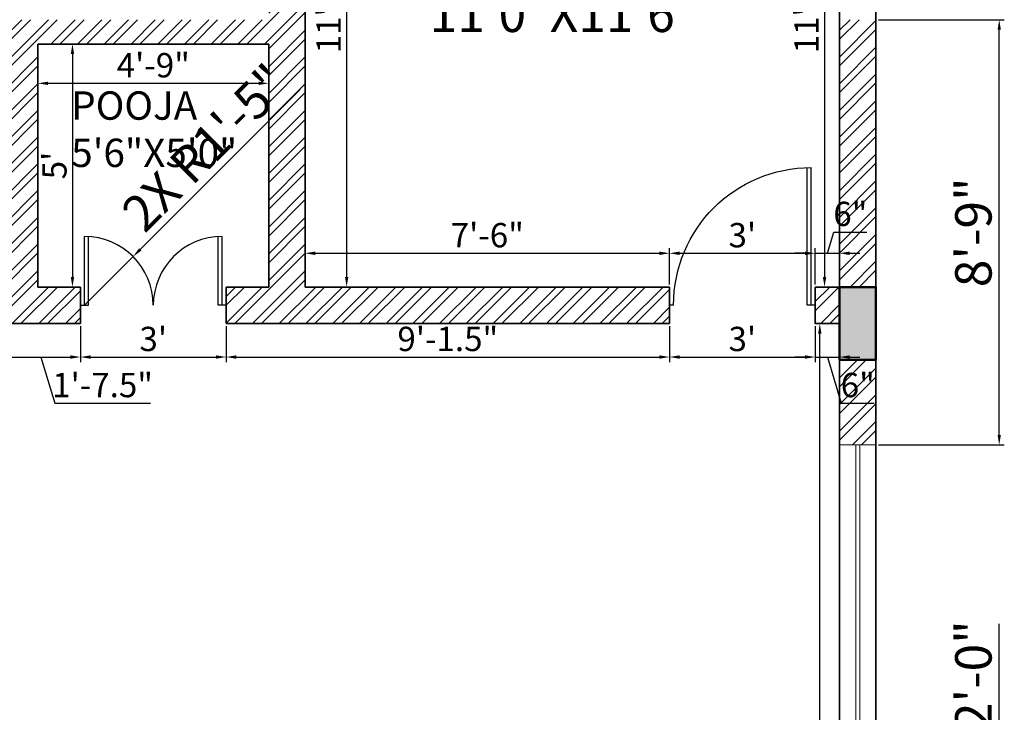
# Model space of a CAD drawing. Units: inches. Extents: x 4153 to 5577, y 785 to 1503.
# Tile 10 of 11: x 5307 to 5550, y 1138 to 1309. Entities that reach past the tile are written whole.
import ezdxf

# ---------------------------------------------------------------- set-up
doc = ezdxf.new("R2010")
doc.units = ezdxf.units.IN
for name, color, linetype, lineweight in [('A-ANNO-DIMS', 2, 'Continuous', 18), ('A-AREA-IDEN', 7, 'Continuous', 25), ('A-COLS', 7, 'Continuous', 50), ('A-DOOR', 3, 'Continuous', 25), ('A-GLAZ', 4, 'Continuous', 18), ('A-WALL', 7, 'Continuous', 35)]:
    doc.layers.add(name, color=color, linetype=linetype, lineweight=lineweight)
doc.layers.add('A-WALL-PATT', color=251, linetype='Continuous', lineweight=13, true_color=0x636466)
doc.styles.get("Standard").update_dxf_attribs({"font": 'arial.ttf'})
doc.dimstyles.new('ISO-25', dxfattribs={"dimtxt": 9, "dimasz": 2.5, "dimexe": 1.25, "dimexo": 0.625, "dimtad": 1, "dimlunit": 3, "dimtxsty": 'Standard', "dimcen": 2.5, "dimadec": 0, "dimazin": 0, "dimtfac": 1, "dimtmove": 0, "dimatfit": 3, "dimfxl": 1, "dimarcsym": 0})

# ---------------------------------------------------------------- blocks, each defined once
blk = doc.blocks.new('D1')
for p, q in [((1, 0), (1, 34)), ((2, 0), (2, 33.99)), ((0, 0), (2, 0)), ((35, 0), (36, 0))]:
    blk.add_line(p, q)
at = {"ltscale": 0.5}
blk.add_arc((1, 0), 34, 0, 90, dxfattribs=at)
blk = doc.blocks.new('D3')
for p, q in [((1, 0), (1, 17)), ((2, 0), (2, 16.97)), ((34, 0), (34, 16.97)), ((35, 0), (35, 17)), ((0, 0), (2, 0)), ((36, 0), (34, 0))]:
    blk.add_line(p, q)
at = {"ltscale": 0.5}
for centre, start, end in [((1, 0), 0, 90), ((35, 0), 90, 180)]:
    blk.add_arc(centre, 17, start, end, dxfattribs=at)
blk = doc.blocks.new('*D58')
at = {"layer": 'A-ANNO-DIMS', "color": 0, "lineweight": -2, "transparency": 16777216}
for p, q in [((5508.63, 1234.49), (5503.13, 1234.49)), ((5504.38, 1002.99), (5504.38, 1231.99)), ((5508.63, 1000.49), (5503.13, 1000.49))]:
    blk.add_line(p, q, dxfattribs=at)
at = {"layer": 'A-ANNO-DIMS', "color": 0, "transparency": 16777216}
for points in [[(5503.97, 1231.99), (5504.8, 1231.99), (5504.38, 1234.49)], [(5503.97, 1002.99), (5504.8, 1002.99), (5504.38, 1000.49)]]:
    blk.add_solid(points, dxfattribs=at)
at = {"layer": 'Defpoints', "color": 0, "transparency": 16777216}
for p in [(5504.38, 1234.49), (5509.25, 1234.49), (5509.25, 1000.49)]:
    blk.add_point(p, dxfattribs=at)
at = {"layer": 'A-ANNO-DIMS', "color": 0, "transparency": 16777216, "insert": (5500.69, 1117.49), "char_height": 6, "attachment_point": 5, "rotation": 90}
blk.add_mtext('19\'-6"', dxfattribs=at)
blk = doc.blocks.new('*D60')
at = {"layer": 'A-ANNO-DIMS', "color": 0, "lineweight": -2, "transparency": 16777216}
for p, q in [((5302.25, 1233.86), (5302.25, 1224.95)), ((5321.75, 1233.86), (5321.75, 1224.95)), ((5304.75, 1226.2), (5319.25, 1226.2)), ((5312, 1226.2), (5315.42, 1214.82)), ((5315.42, 1214.82), (5339.04, 1214.82))]:
    blk.add_line(p, q, dxfattribs=at)
at = {"layer": 'A-ANNO-DIMS', "color": 0, "transparency": 16777216}
for points in [[(5304.75, 1226.62), (5304.75, 1225.78), (5302.25, 1226.2)], [(5319.25, 1226.62), (5319.25, 1225.78), (5321.75, 1226.2)]]:
    blk.add_solid(points, dxfattribs=at)
at = {"layer": 'Defpoints', "color": 0, "transparency": 16777216}
for p in [(5302.25, 1234.49), (5321.75, 1234.49), (5321.75, 1226.2)]:
    blk.add_point(p, dxfattribs=at)
at = {"layer": 'A-ANNO-DIMS', "color": 0, "transparency": 16777216, "insert": (5327.23, 1218.51), "char_height": 6, "attachment_point": 5}
blk.add_mtext('1\'-7.5"', dxfattribs=at)
blk = doc.blocks.new('*D61')
at = {"layer": 'A-ANNO-DIMS', "color": 0, "lineweight": -2, "transparency": 16777216}
for p, q in [((5321.75, 1233.86), (5321.75, 1224.95)), ((5357.75, 1233.86), (5357.75, 1224.95)), ((5324.25, 1226.2), (5355.25, 1226.2))]:
    blk.add_line(p, q, dxfattribs=at)
at = {"layer": 'A-ANNO-DIMS', "color": 0, "transparency": 16777216}
for points in [[(5324.25, 1226.62), (5324.25, 1225.78), (5321.75, 1226.2)], [(5355.25, 1226.62), (5355.25, 1225.78), (5357.75, 1226.2)]]:
    blk.add_solid(points, dxfattribs=at)
at = {"layer": 'Defpoints', "color": 0, "transparency": 16777216}
for p in [(5321.75, 1234.49), (5357.75, 1234.49), (5357.75, 1226.2)]:
    blk.add_point(p, dxfattribs=at)
at = {"layer": 'A-ANNO-DIMS', "color": 0, "transparency": 16777216, "insert": (5339.75, 1229.89), "char_height": 6, "attachment_point": 5}
blk.add_mtext("3'", dxfattribs=at)
blk = doc.blocks.new('*D62')
at = {"layer": 'A-ANNO-DIMS', "color": 0, "lineweight": -2, "transparency": 16777216}
for p, q in [((5357.75, 1233.86), (5357.75, 1224.95)), ((5467.25, 1233.86), (5467.25, 1224.95)), ((5360.25, 1226.2), (5464.75, 1226.2))]:
    blk.add_line(p, q, dxfattribs=at)
at = {"layer": 'A-ANNO-DIMS', "color": 0, "transparency": 16777216}
for points in [[(5360.25, 1226.62), (5360.25, 1225.78), (5357.75, 1226.2)], [(5464.75, 1226.62), (5464.75, 1225.78), (5467.25, 1226.2)]]:
    blk.add_solid(points, dxfattribs=at)
at = {"layer": 'Defpoints', "color": 0, "transparency": 16777216}
for p in [(5357.75, 1234.49), (5467.25, 1234.49), (5467.25, 1226.2)]:
    blk.add_point(p, dxfattribs=at)
at = {"layer": 'A-ANNO-DIMS', "color": 0, "transparency": 16777216, "insert": (5412.5, 1229.89), "char_height": 6, "attachment_point": 5}
blk.add_mtext('9\'-1.5"', dxfattribs=at)
blk = doc.blocks.new('*D63')
at = {"layer": 'A-ANNO-DIMS', "color": 0, "lineweight": -2, "transparency": 16777216}
for p, q in [((5467.25, 1233.86), (5467.25, 1224.95)), ((5503.25, 1233.86), (5503.25, 1224.95)), ((5469.75, 1226.2), (5500.75, 1226.2))]:
    blk.add_line(p, q, dxfattribs=at)
at = {"layer": 'A-ANNO-DIMS', "color": 0, "transparency": 16777216}
for points in [[(5469.75, 1226.62), (5469.75, 1225.78), (5467.25, 1226.2)], [(5500.75, 1226.62), (5500.75, 1225.78), (5503.25, 1226.2)]]:
    blk.add_solid(points, dxfattribs=at)
at = {"layer": 'Defpoints', "color": 0, "transparency": 16777216}
for p in [(5467.25, 1234.49), (5503.25, 1234.49), (5503.25, 1226.2)]:
    blk.add_point(p, dxfattribs=at)
at = {"layer": 'A-ANNO-DIMS', "color": 0, "transparency": 16777216, "insert": (5485.25, 1229.89), "char_height": 6, "attachment_point": 5}
blk.add_mtext("3'", dxfattribs=at)
blk = doc.blocks.new('*D64')
at = {"layer": 'A-ANNO-DIMS', "color": 0, "lineweight": -2, "transparency": 16777216}
for p, q in [((5503.25, 1233.86), (5503.25, 1224.95)), ((5509.25, 1233.86), (5509.25, 1224.95)), ((5500.75, 1226.2), (5498.25, 1226.2)), ((5503.25, 1226.2), (5509.25, 1226.2)), ((5503.25, 1226.2), (5509.25, 1226.2)), ((5506.25, 1226.2), (5509.67, 1214.82)), ((5511.75, 1226.2), (5514.25, 1226.2)), ((5509.67, 1214.82), (5517.85, 1214.82))]:
    blk.add_line(p, q, dxfattribs=at)
at = {"layer": 'A-ANNO-DIMS', "color": 0, "transparency": 16777216}
for points in [[(5500.75, 1226.62), (5500.75, 1225.78), (5503.25, 1226.2)], [(5511.75, 1226.62), (5511.75, 1225.78), (5509.25, 1226.2)]]:
    blk.add_solid(points, dxfattribs=at)
at = {"layer": 'Defpoints', "color": 0, "transparency": 16777216}
for p in [(5503.25, 1234.49), (5509.25, 1234.49), (5509.25, 1226.2)]:
    blk.add_point(p, dxfattribs=at)
at = {"layer": 'A-ANNO-DIMS', "color": 0, "transparency": 16777216, "insert": (5513.76, 1218.51), "char_height": 6, "attachment_point": 5}
blk.add_mtext('6"', dxfattribs=at)
blk = doc.blocks.new('*D65')
at = {"layer": 'A-ANNO-DIMS', "color": 0, "lineweight": -2, "transparency": 16777216}
for p, q in [((5311.88, 1303.49), (5321.03, 1303.49)), ((5319.78, 1300.99), (5319.78, 1245.99)), ((5311.88, 1243.49), (5321.03, 1243.49))]:
    blk.add_line(p, q, dxfattribs=at)
at = {"layer": 'A-ANNO-DIMS', "color": 0, "transparency": 16777216}
for points in [[(5319.37, 1300.99), (5320.2, 1300.99), (5319.78, 1303.49)], [(5319.37, 1245.99), (5320.2, 1245.99), (5319.78, 1243.49)]]:
    blk.add_solid(points, dxfattribs=at)
at = {"layer": 'Defpoints', "color": 0, "transparency": 16777216}
for p in [(5311.25, 1303.49), (5311.25, 1243.49), (5319.78, 1243.49)]:
    blk.add_point(p, dxfattribs=at)
at = {"layer": 'A-ANNO-DIMS', "color": 0, "transparency": 16777216, "insert": (5316.11, 1273.49), "char_height": 6, "attachment_point": 5, "rotation": 90}
blk.add_mtext("5'", dxfattribs=at)
blk = doc.blocks.new('*D66')
at = {"layer": 'A-ANNO-DIMS', "color": 0, "lineweight": -2, "transparency": 16777216}
for p, q in [((5311.25, 1302.86), (5311.25, 1292.53)), ((5368.25, 1302.86), (5368.25, 1292.53)), ((5313.75, 1293.78), (5365.75, 1293.78))]:
    blk.add_line(p, q, dxfattribs=at)
at = {"layer": 'A-ANNO-DIMS', "color": 0, "transparency": 16777216}
for points in [[(5313.75, 1294.19), (5313.75, 1293.36), (5311.25, 1293.78)], [(5365.75, 1294.19), (5365.75, 1293.36), (5368.25, 1293.78)]]:
    blk.add_solid(points, dxfattribs=at)
at = {"layer": 'Defpoints', "color": 0, "transparency": 16777216}
for p in [(5311.25, 1303.49), (5368.25, 1303.49), (5368.25, 1293.78)]:
    blk.add_point(p, dxfattribs=at)
at = {"layer": 'A-ANNO-DIMS', "color": 0, "transparency": 16777216, "insert": (5339.75, 1297.47), "char_height": 6, "attachment_point": 5}
blk.add_mtext('4\'-9"', dxfattribs=at)
blk = doc.blocks.new('*D67')
at = {"layer": 'A-ANNO-DIMS', "color": 0, "lineweight": -2, "transparency": 16777216}
for p, q in [((5377.88, 1381.49), (5388.77, 1381.49)), ((5387.52, 1245.99), (5387.52, 1378.99)), ((5377.88, 1243.49), (5388.77, 1243.49))]:
    blk.add_line(p, q, dxfattribs=at)
at = {"layer": 'A-ANNO-DIMS', "color": 0, "transparency": 16777216}
for points in [[(5387.1, 1378.99), (5387.94, 1378.99), (5387.52, 1381.49)], [(5387.1, 1245.99), (5387.94, 1245.99), (5387.52, 1243.49)]]:
    blk.add_solid(points, dxfattribs=at)
at = {"layer": 'Defpoints', "color": 0, "transparency": 16777216}
for p in [(5377.25, 1381.49), (5387.52, 1381.49), (5377.25, 1243.49)]:
    blk.add_point(p, dxfattribs=at)
at = {"layer": 'A-ANNO-DIMS', "color": 0, "transparency": 16777216, "insert": (5383.83, 1312.49), "char_height": 6, "attachment_point": 5, "rotation": 90}
blk.add_mtext('11\'-6"', dxfattribs=at)
blk = doc.blocks.new('*D68')
at = {"layer": 'A-ANNO-DIMS', "color": 0, "lineweight": -2, "transparency": 16777216}
for p, q in [((5377.25, 1244.11), (5377.25, 1253.07)), ((5467.25, 1244.11), (5467.25, 1253.07)), ((5379.75, 1251.82), (5464.75, 1251.82))]:
    blk.add_line(p, q, dxfattribs=at)
at = {"layer": 'A-ANNO-DIMS', "color": 0, "transparency": 16777216}
for points in [[(5379.75, 1252.24), (5379.75, 1251.4), (5377.25, 1251.82)], [(5464.75, 1252.24), (5464.75, 1251.4), (5467.25, 1251.82)]]:
    blk.add_solid(points, dxfattribs=at)
at = {"layer": 'Defpoints', "color": 0, "transparency": 16777216}
for p in [(5467.25, 1251.82), (5377.25, 1243.49), (5467.25, 1243.49)]:
    blk.add_point(p, dxfattribs=at)
at = {"layer": 'A-ANNO-DIMS', "color": 0, "transparency": 16777216, "insert": (5422.25, 1255.51), "char_height": 6, "attachment_point": 5}
blk.add_mtext('7\'-6"', dxfattribs=at)
blk = doc.blocks.new('*D69')
at = {"layer": 'A-ANNO-DIMS', "color": 0, "lineweight": -2, "transparency": 16777216}
for p, q in [((5467.25, 1244.11), (5467.25, 1253.07)), ((5503.25, 1244.11), (5503.25, 1253.07)), ((5469.75, 1251.82), (5500.75, 1251.82))]:
    blk.add_line(p, q, dxfattribs=at)
at = {"layer": 'A-ANNO-DIMS', "color": 0, "transparency": 16777216}
for points in [[(5469.75, 1252.24), (5469.75, 1251.4), (5467.25, 1251.82)], [(5500.75, 1252.24), (5500.75, 1251.4), (5503.25, 1251.82)]]:
    blk.add_solid(points, dxfattribs=at)
at = {"layer": 'Defpoints', "color": 0, "transparency": 16777216}
for p in [(5503.25, 1251.82), (5467.25, 1243.49), (5503.25, 1243.49)]:
    blk.add_point(p, dxfattribs=at)
at = {"layer": 'A-ANNO-DIMS', "color": 0, "transparency": 16777216, "insert": (5485.25, 1255.51), "char_height": 6, "attachment_point": 5}
blk.add_mtext("3'", dxfattribs=at)
blk = doc.blocks.new('*D70')
at = {"layer": 'A-ANNO-DIMS', "color": 0, "lineweight": -2, "transparency": 16777216}
for p, q in [((5506.25, 1251.82), (5507.83, 1257.07)), ((5507.83, 1257.07), (5516.01, 1257.07)), ((5503.25, 1244.11), (5503.25, 1253.07)), ((5509.25, 1244.11), (5509.25, 1253.07)), ((5500.75, 1251.82), (5498.25, 1251.82)), ((5503.25, 1251.82), (5509.25, 1251.82)), ((5503.25, 1251.82), (5509.25, 1251.82)), ((5511.75, 1251.82), (5514.25, 1251.82))]:
    blk.add_line(p, q, dxfattribs=at)
at = {"layer": 'A-ANNO-DIMS', "color": 0, "transparency": 16777216}
for points in [[(5500.75, 1252.24), (5500.75, 1251.4), (5503.25, 1251.82)], [(5511.75, 1252.24), (5511.75, 1251.4), (5509.25, 1251.82)]]:
    blk.add_solid(points, dxfattribs=at)
at = {"layer": 'Defpoints', "color": 0, "transparency": 16777216}
for p in [(5509.25, 1251.82), (5503.25, 1243.49), (5509.25, 1243.49)]:
    blk.add_point(p, dxfattribs=at)
at = {"layer": 'A-ANNO-DIMS', "color": 0, "transparency": 16777216, "insert": (5511.92, 1260.76), "char_height": 6, "attachment_point": 5}
blk.add_mtext('6"', dxfattribs=at)
blk = doc.blocks.new('*D82')
at = {"layer": 'A-ANNO-DIMS', "color": 0, "lineweight": -2, "transparency": 16777216}
for p, q in [((5508.63, 1381.49), (5504.31, 1381.49)), ((5505.56, 1378.99), (5505.56, 1245.99)), ((5508.63, 1243.49), (5504.31, 1243.49))]:
    blk.add_line(p, q, dxfattribs=at)
at = {"layer": 'A-ANNO-DIMS', "color": 0, "transparency": 16777216}
for points in [[(5505.14, 1378.99), (5505.97, 1378.99), (5505.56, 1381.49)], [(5505.14, 1245.99), (5505.97, 1245.99), (5505.56, 1243.49)]]:
    blk.add_solid(points, dxfattribs=at)
at = {"layer": 'Defpoints', "color": 0, "transparency": 16777216}
for p in [(5509.25, 1381.49), (5505.56, 1243.49), (5509.25, 1243.49)]:
    blk.add_point(p, dxfattribs=at)
at = {"layer": 'A-ANNO-DIMS', "color": 0, "transparency": 16777216, "insert": (5501.87, 1312.49), "char_height": 6, "attachment_point": 5, "rotation": 90}
blk.add_mtext('11\'-6"', dxfattribs=at)
blk = doc.blocks.new('WINDOW-72IN')
for p, q in [((0, 9), (0, 0)), ((72, 9), (72, 0)), ((0, 5), (72, 5)), ((0, 4), (72, 4))]:
    blk.add_line(p, q)
blk = doc.blocks.new('COL-9X18IN')
at = {"transparency": 33554687}
h = blk.add_hatch(color=256, dxfattribs=at)
h.dxf.hatch_style = 1
h.paths.add_polyline_path([(9, 18), (0, 18), (0, 0), (9, 0)])
blk.add_lwpolyline([(0, 18), (9, 18), (9, 0), (0, 0)], close=True)
blk = doc.blocks.new('*D154')
at = {"layer": 'A-ANNO-DIMS', "color": 0, "lineweight": -2, "transparency": 16777216}
for p, q in [((5548.7, 1132.49), (5548.7, 1160.32)), ((5518.88, 1132.49), (5549.95, 1132.49)), ((5548.7, 1110.99), (5548.7, 1129.99)), ((5518.88, 1108.49), (5549.95, 1108.49))]:
    blk.add_line(p, q, dxfattribs=at)
at = {"layer": 'A-ANNO-DIMS', "color": 0, "transparency": 16777216}
for points in [[(5548.29, 1129.99), (5549.12, 1129.99), (5548.7, 1132.49)], [(5548.29, 1110.99), (5549.12, 1110.99), (5548.7, 1108.49)]]:
    blk.add_solid(points, dxfattribs=at)
at = {"layer": 'Defpoints', "color": 0, "transparency": 16777216}
for p in [(5518.25, 1132.49), (5548.7, 1132.49), (5518.25, 1108.49)]:
    blk.add_point(p, dxfattribs=at)
at = {"layer": 'A-ANNO-DIMS', "color": 0, "transparency": 16777216, "insert": (5543.48, 1147.65), "char_height": 9, "attachment_point": 5, "rotation": 90}
blk.add_mtext('2\'-0"', dxfattribs=at)
blk = doc.blocks.new('*D155')
at = {"layer": 'A-ANNO-DIMS', "color": 0, "lineweight": -2, "transparency": 16777216}
for p, q in [((5518.88, 1309.49), (5549.95, 1309.49)), ((5548.7, 1206.99), (5548.7, 1306.99)), ((5518.88, 1204.49), (5549.95, 1204.49))]:
    blk.add_line(p, q, dxfattribs=at)
at = {"layer": 'A-ANNO-DIMS', "color": 0, "transparency": 16777216}
for points in [[(5548.29, 1306.99), (5549.12, 1306.99), (5548.7, 1309.49)], [(5548.29, 1206.99), (5549.12, 1206.99), (5548.7, 1204.49)]]:
    blk.add_solid(points, dxfattribs=at)
at = {"layer": 'Defpoints', "color": 0, "transparency": 16777216}
for p in [(5518.25, 1309.49), (5548.7, 1309.49), (5518.25, 1204.49)]:
    blk.add_point(p, dxfattribs=at)
at = {"layer": 'A-ANNO-DIMS', "color": 0, "transparency": 16777216, "insert": (5543.48, 1256.99), "char_height": 9, "attachment_point": 5, "rotation": 90}
blk.add_mtext('8\'-9"', dxfattribs=at)
blk = doc.blocks.new('*D163')
at = {"layer": 'A-ANNO-DIMS', "color": 0, "lineweight": -2, "transparency": 16777216}
for p, q in [((5375.99, 1292.22), (5336.54, 1252.78)), ((5322.75, 1238.99), (5334.77, 1251.01))]:
    blk.add_line(p, q, dxfattribs=at)
at = {"layer": 'A-ANNO-DIMS', "color": 0, "transparency": 16777216}
blk.add_solid([(5336.25, 1253.07), (5336.84, 1252.48), (5334.77, 1251.01)], dxfattribs=at)
at = {"layer": 'Defpoints', "color": 0, "transparency": 16777216}
for p in [(5334.77, 1251.01), (5322.75, 1238.99)]:
    blk.add_point(p, dxfattribs=at)
at = {"layer": 'A-ANNO-DIMS', "color": 0, "transparency": 16777216, "insert": (5353.46, 1277.07), "char_height": 9, "attachment_point": 5, "rotation": 44.9986}
blk.add_mtext('2X R1\'-5"', dxfattribs=at)

msp = doc.modelspace()

# ---------------------------------------------------------------- hatches: boundary and pattern name
at = {"layer": 'A-WALL-PATT', "transparency": 33554687}
h = msp.add_hatch(dxfattribs=at)
h.set_pattern_fill('ANSI32', color=256, scale=0.49)
h.set_pattern_definition([(45, (816.3263, 0), (-3.300244, 3.300244), []), (45, (818.5265, 0), (-3.300244, 3.300244), [])])
h.paths.add_polyline_path([(5011.254, 1088.988), (5020.254, 1088.988), (5020.254, 1129.488), (5155.254, 1129.488), (5155.254, 1105.488), (5161.254, 1105.488), (5161.254, 1138.488), (5098.254, 1138.488), (5098.254, 1234.488), (5113.254, 1234.488), (5113.254, 1243.488), (5086.254, 1243.488), (5086.254, 1234.488), (5092.254, 1234.488), (5092.254, 1138.488), (5020.254, 1138.488), (5020.254, 1168.488), (5011.254, 1168.488)])
h.paths.add_polyline_path([(5011.254, 1009.488), (5020.254, 1009.488), (5020.254, 1040.988), (5011.254, 1040.988)])
h.paths.add_polyline_path([(5095.254, 991.488), (5095.254, 1000.488), (5020.254, 1000.488), (5020.254, 991.488)])
h.paths.add_polyline_path([(5011.254, 910.488), (5020.254, 910.488), (5020.254, 991.488), (5011.254, 991.488)])
h.paths.add_polyline_path([(5152.254, 901.488), (5152.254, 907.488), (5020.254, 907.488), (5020.254, 901.488)])
h.paths.add_polyline_path([(5161.254, 1057.488), (5155.254, 1057.488), (5155.254, 1000.488), (5161.254, 1000.488)])
h.paths.add_polyline_path([(5143.254, 991.488), (5152.254, 991.488), (5152.254, 1000.488), (5143.254, 1000.488)])
h.paths.add_polyline_path([(5161.254, 1000.488), (5161.254, 991.488), (5185.254, 991.488), (5185.254, 1000.488)])
h.paths.add_polyline_path([(5257.254, 991.488), (5257.254, 1000.488), (5233.254, 1000.488), (5233.254, 991.488)])
h.paths.add_polyline_path([(5266.254, 1120.488), (5257.254, 1120.488), (5257.254, 1000.488), (5266.254, 1000.488)])
h.paths.add_polyline_path([(5290.254, 991.488), (5290.254, 1000.488), (5275.254, 1000.488), (5275.254, 991.488)])
h.paths.add_polyline_path([(5362.254, 1000.488), (5362.254, 991.488), (5455.254, 991.488), (5455.254, 1000.488)])
h.paths.add_polyline_path([(5509.254, 1009.488), (5518.254, 1009.488), (5518.254, 1036.488), (5509.254, 1036.488)])
h.paths.add_polyline_path([(5503.254, 1000.488), (5503.254, 991.488), (5509.254, 991.488), (5509.254, 1000.488)])
h.paths.add_polyline_path([(5518.254, 1132.488), (5509.254, 1132.488), (5509.254, 1108.488), (5518.254, 1108.488)])
h.paths.add_polyline_path([(5509.254, 1204.488), (5518.254, 1204.488), (5518.254, 1225.488), (5509.254, 1225.488)])
h.paths.add_polyline_path([(5467.254, 1234.488), (5467.254, 1243.488), (5377.254, 1243.488), (5377.254, 1265.228), (5377.254, 1381.488), (5467.254, 1381.488), (5467.254, 1393.488), (5461.254, 1393.488), (5461.254, 1387.488), (5377.254, 1387.488), (5377.254, 1435.488), (5368.254, 1435.488), (5368.254, 1354.488), (5347.254, 1354.488), (5347.254, 1348.488), (5368.254, 1348.488), (5368.254, 1309.488), (5302.254, 1309.488), (5302.254, 1234.488), (5321.754, 1234.488), (5321.754, 1243.488), (5311.254, 1243.488), (5311.254, 1303.488), (5368.254, 1303.488), (5368.254, 1243.488), (5357.754, 1243.488), (5357.754, 1234.488)])
h.paths.add_polyline_path([(5509.254, 1357.488), (5518.254, 1357.488), (5518.254, 1426.488), (5509.254, 1426.488)])
h.paths.add_polyline_path([(5509.254, 1243.488), (5518.254, 1243.488), (5518.254, 1309.488), (5509.254, 1309.488)])
h.paths.add_polyline_path([(5509.254, 1435.488), (5509.254, 1444.488), (5425.254, 1444.488), (5425.254, 1435.488), (5461.254, 1435.488), (5461.254, 1423.488), (5467.254, 1423.488), (5467.254, 1435.488)])
h.paths.add_polyline_path([(5302.254, 1435.488), (5302.254, 1348.488), (5317.254, 1348.488), (5317.254, 1354.488), (5311.254, 1354.488), (5311.254, 1435.488), (5314.254, 1435.488), (5314.254, 1444.488), (5296.254, 1444.488), (5296.254, 1435.488)])
h.paths.add_polyline_path([(5368.254, 1444.488), (5362.254, 1444.488), (5362.254, 1435.488), (5368.254, 1435.488)])
h.paths.add_polyline_path([(5389.254, 1444.488), (5386.254, 1444.488), (5386.254, 1435.488), (5389.254, 1435.488)])
h.paths.add_polyline_path([(5248.254, 1435.488), (5248.254, 1444.488), (5173.254, 1444.488), (5173.254, 1435.488)])
h.paths.add_polyline_path([(5101.254, 1435.488), (5101.254, 1444.488), (5020.254, 1444.488), (5020.254, 1435.488)])
h.paths.add_polyline_path([(5011.254, 1293.488), (5020.254, 1293.488), (5020.254, 1295.242), (5020.254, 1426.488), (5011.254, 1426.488)])
h.paths.add_polyline_path([(5155.254, 1243.488), (5149.254, 1243.488), (5149.254, 1234.488), (5248.254, 1234.488), (5248.254, 1243.488), (5164.254, 1243.488), (5164.254, 1435.488), (5155.254, 1435.488)])
h.paths.add_polyline_path([(5020.254, 1243.488), (5020.254, 1234.488), (5056.254, 1234.488), (5056.254, 1243.488)], flags=17)
h.paths.add_polyline_path([(5020.254, 1225.488), (5011.254, 1225.488), (5011.254, 1198.488), (5020.254, 1198.488)], flags=17)
h = msp.add_hatch(dxfattribs=at)
h.set_pattern_fill('ANSI32', color=256, scale=0.5)
h.paths.add_polyline_path([(5509.254, 1243.488), (5503.254, 1243.488), (5503.254, 1234.488), (5509.254, 1234.488)])

# ---------------------------------------------------------------- linework, layer by layer
at = {"layer": 'A-WALL'}
for p, q in [((5518.254, 1444.488), (5518.254, 901.488)), ((5509.254, 1435.488), (5509.254, 1243.488)), ((5377.254, 1243.488), (5377.254, 1381.488)), ((5311.254, 1303.488), (5368.254, 1303.488)), ((5311.254, 1243.488), (5311.254, 1303.488)), ((5368.254, 1243.488), (5368.254, 1303.488)), ((5311.254, 1243.488), (5321.754, 1243.488)), ((5321.754, 1243.488), (5321.754, 1234.488)), ((5357.754, 1243.488), (5368.254, 1243.488)), ((5357.754, 1243.488), (5357.754, 1234.488)), ((5377.254, 1243.488), (5467.254, 1243.488)), ((5467.254, 1243.488), (5467.254, 1234.488)), ((5503.254, 1243.488), (5509.254, 1243.488)), ((5503.254, 1243.488), (5503.254, 1234.488)), ((5302.254, 1234.488), (5321.754, 1234.488)), ((5357.754, 1234.488), (5467.254, 1234.488)), ((5503.254, 1234.488), (5509.254, 1234.488)), ((5509.254, 1234.488), (5509.254, 1000.488))]:
    msp.add_line(p, q, dxfattribs=at)

# ---------------------------------------------------------------- block references
at = {"layer": 'A-COLS'}
msp.add_blockref('COL-9X18IN', (5509.254, 1225.488), dxfattribs=at)
at = {"layer": 'A-DOOR', "xscale": -1}
msp.add_blockref('D1', (5503.254, 1238.988), dxfattribs=at)
at = {"layer": 'A-DOOR'}
msp.add_blockref('D3', (5321.754, 1238.988), dxfattribs=at)
at = {"layer": 'A-GLAZ', "rotation": 269.9999999999994}
msp.add_blockref('WINDOW-72IN', (5509.254, 1204.488), dxfattribs=at)

# ---------------------------------------------------------------- texts
at = {"layer": 'A-AREA-IDEN', "attachment_point": 1}
for s, heights, insert, char_height in [('{\\fTimes New Roman|b0|i0|c0|p18;BEDROOM\\P11\'0"X11\'6"}', [0], (5407.994, 1330.447), 9), ('{\\fTimes New Roman|b0|i0|c0|p18;POOJA\\P5\'6"X5\'0"}', [18.808], (5319.482, 1291.789), 7)]:
    msp.add_mtext_dynamic_manual_height_columns(s, width=67.35079, gutter_width=12.5, heights=heights, dxfattribs=dict(at, insert=insert, char_height=char_height))

# ---------------------------------------------------------------- dimensions: what is measured, and where the dimension line sits
at = {"layer": 'A-ANNO-DIMS'}
for base, p1, p2, override, picture, middle in [((5387.52, 1381.488), (5377.254, 1243.488), (5377.254, 1381.488), {"dimtxt": 6, "dimclrd": 0, "dimclre": 0, "dimclrt": 0}, '*D67', (5383.832, 1312.488)), ((5505.555, 1243.488), (5509.254, 1381.488), (5509.254, 1243.488), {"dimtxt": 6, "dimclrd": 0, "dimclre": 0, "dimclrt": 0}, '*D82', (5501.867, 1312.488)), ((5548.704, 1309.488), (5518.254, 1204.488), (5518.254, 1309.488), {"dimdec": 1, "dimlfac": 1, "dimrnd": 0, "dimzin": 1, "dimdsep": 46, "dimlunit": 4, "dimfrac": 2}, '*D155', (5543.484, 1256.988)), ((5319.783, 1243.488), (5311.254, 1303.488), (5311.254, 1243.488), {"dimtxt": 6, "dimclrd": 0, "dimclre": 0, "dimclrt": 0}, '*D65', (5316.107, 1273.488)), ((5504.382, 1234.488), (5509.254, 1000.488), (5509.254, 1234.488), {"dimtxt": 6, "dimclrd": 0, "dimclre": 0, "dimclrt": 0}, '*D58', (5500.693, 1117.488)), ((5548.704, 1132.488), (5518.254, 1108.488), (5518.254, 1132.488), {"dimdec": 1, "dimlfac": 1, "dimrnd": 0, "dimzin": 1, "dimdsep": 46, "dimlunit": 4, "dimfrac": 2}, '*D154', (5543.484, 1147.652))]:
    dim = msp.add_linear_dim(base=base, p1=p1, p2=p2, angle=90, dimstyle='ISO-25', override=override, dxfattribs=at)
    dim.commit()
    dim.dimension.update_dxf_attribs({"geometry": picture, "text_midpoint": middle})
for base, p1, p2, override, picture, middle in [((5368.254, 1293.778), (5311.254, 1303.488), (5368.254, 1303.488), {"dimtxt": 6, "dimclrd": 0, "dimclre": 0, "dimclrt": 0}, '*D66', (5339.754, 1297.466)), ((5509.254, 1251.819), (5503.254, 1243.488), (5509.254, 1243.488), {"dimtxt": 6, "dimclrd": 0, "dimclre": 0, "dimclrt": 0, "dimtmove": 1}, '*D70', (5508.454, 1260.758)), ((5467.254, 1251.819), (5377.254, 1243.488), (5467.254, 1243.488), {"dimtxt": 6, "dimclrd": 0, "dimclre": 0, "dimclrt": 0}, '*D68', (5422.254, 1255.507)), ((5503.254, 1251.819), (5467.254, 1243.488), (5503.254, 1243.488), {"dimtxt": 6, "dimclrd": 0, "dimclre": 0, "dimclrt": 0, "dimtmove": 1}, '*D69', (5485.254, 1255.509)), ((5321.754, 1226.199), (5302.254, 1234.488), (5321.754, 1234.488), {"dimtxt": 6, "dimclrd": 0, "dimclre": 0, "dimclrt": 0, "dimtmove": 1}, '*D60', (5316.042, 1218.51)), ((5357.754, 1226.199), (5321.754, 1234.488), (5357.754, 1234.488), {"dimtxt": 6, "dimclrd": 0, "dimclre": 0, "dimclrt": 0, "dimtmove": 1}, '*D61', (5339.754, 1229.89)), ((5467.254, 1226.199), (5357.754, 1234.488), (5467.254, 1234.488), {"dimtxt": 6, "dimclrd": 0, "dimclre": 0, "dimclrt": 0, "dimtmove": 1}, '*D62', (5412.504, 1229.888)), ((5503.254, 1226.199), (5467.254, 1234.488), (5503.254, 1234.488), {"dimtxt": 6, "dimclrd": 0, "dimclre": 0, "dimclrt": 0, "dimtmove": 1}, '*D63', (5485.254, 1229.89)), ((5509.254, 1226.199), (5503.254, 1234.488), (5509.254, 1234.488), {"dimtxt": 6, "dimclrd": 0, "dimclre": 0, "dimclrt": 0, "dimtmove": 1}, '*D64', (5510.292, 1218.51))]:
    dim = msp.add_linear_dim(base=base, p1=p1, p2=p2, dimstyle='ISO-25', override=override, dxfattribs=at)
    dim.commit()
    dim.dimension.update_dxf_attribs({"geometry": picture, "text_midpoint": middle})
dim = msp.add_radius_dim(center=(5322.754, 1238.988), mpoint=(5334.775, 1251.009), text='2X <>', dimstyle='ISO-25', override={"dimdec": 1, "dimlfac": 1, "dimrnd": 0, "dimzin": 1, "dimdsep": 46, "dimlunit": 4, "dimfrac": 2}, dxfattribs=at)
dim.commit()
dim.dimension.update_dxf_attribs({"geometry": '*D163', "text_midpoint": (5353.457, 1277.072)})

doc.saveas('drawing.dxf')
